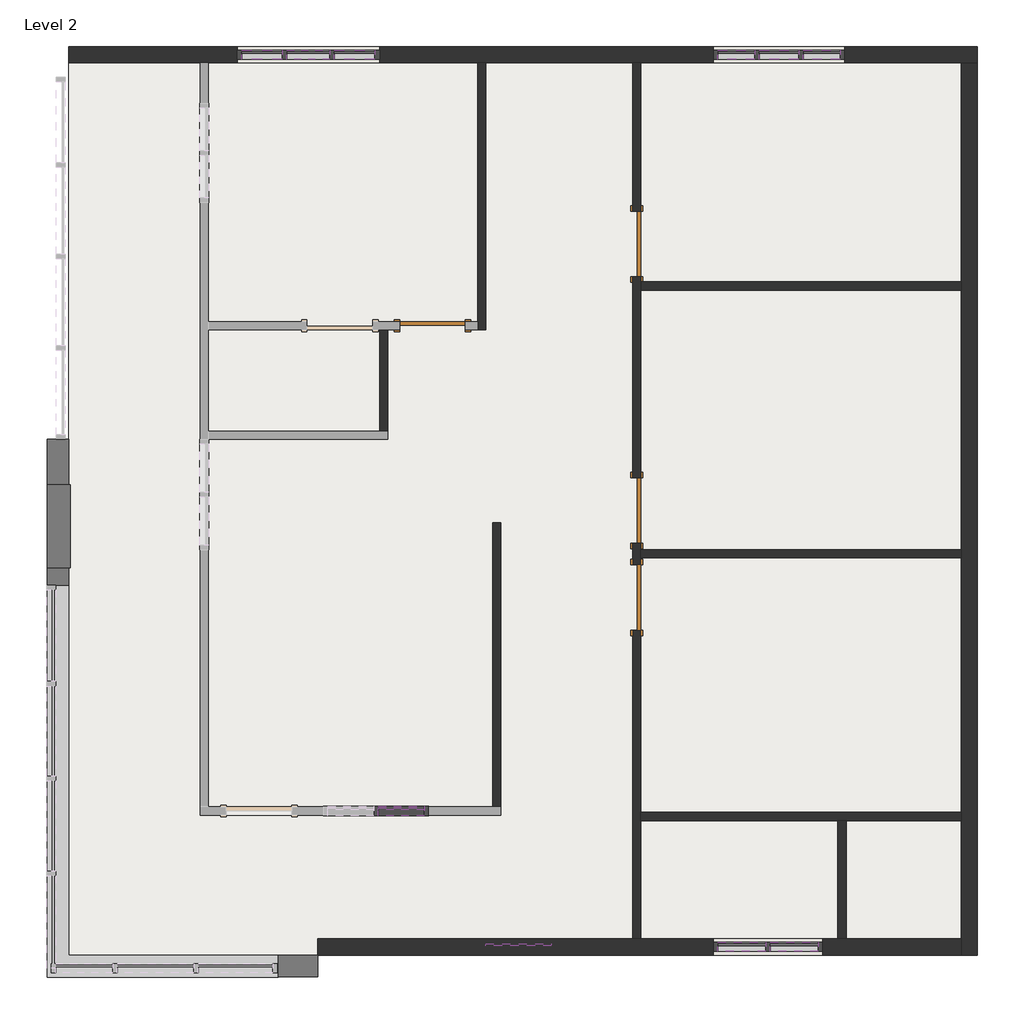
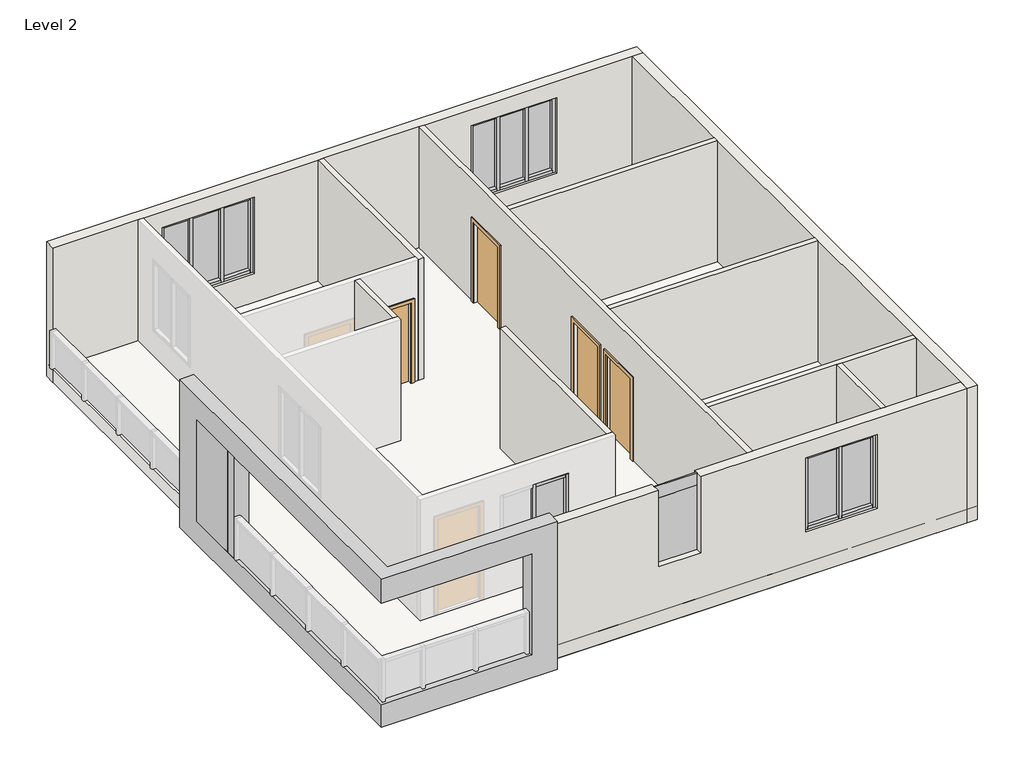
# One storey, part 2 of 2: 31 members, 11 plates, 11 walls, 4 doors, 1 proxy, 1 roof.
"""IFC4 building model written with IfcOpenShell, lengths in millimetres."""

from ifc_helpers import new_model, si_unit, frame, origin, place, context, project, spatial, polyline, outline, extrude, faceted_brep, transform, mapped, element, save
from components import generic_models_2_generic_models_2_8568020c, door_305aa2a5, door_e5f9f3c4, member_0b7646a3, member_a400357f, member_04adda39, member_21317375, member_6ffa5180, member_a980948f, member_e59d77c9, member_427039da, member_6f432376, member_fceb641e, member_70523b0d, member_c33c434a, member_3b0b484b, member_6d86f51b, system_panel_glazed_d508df5b, system_panel_glazed_080605c3, system_panel_glazed_66fd639c, system_panel_glazed_47f9b868, system_panel_glazed_7d7b3bbd, system_panel_glazed_3397605a, system_panel_glazed_23092caa, system_panel_glazed_25c2e5f5

model = new_model("IFC4")

# Units and contexts
model_context = context("Model", 3, world=origin())
ifc_project = project(units=[si_unit("LENGTHUNIT", "METRE", prefix="MILLI")], contexts=[model_context])

# Site, building, storey
site = spatial("IfcSite", under=ifc_project)
building = spatial("IfcBuilding", under=site)
storey = spatial("IfcBuildingStorey", under=building, Name="Level 2", Elevation=3048.0)

# Proxy
placement = place(None, origin())
generic_models_2_generic_models_2_shape = generic_models_2_generic_models_2_8568020c(model_context)
element("IfcBuildingElementProxy", 1, Name="Generic Models 2 : Generic Models 2", ObjectType="Generic Models 2 : Generic Models 2", at=placement, inside=storey, context=model_context, shape_type="MappedRepresentation", body=[
    mapped(generic_models_2_generic_models_2_shape, transform((0.0, 0.0, 0.0), x_axis=(1.0, 0.0, 0.0), y_axis=(0.0, 1.0, 0.0), z_axis=(0.0, 0.0, 1.0))),
])

# Doors
door_shape = door_305aa2a5(model_context)
element("IfcDoor", 2, ObjectType="Single-Flush : 36\" x 84\"", at=placement, inside=storey, context=model_context, shape_type="MappedRepresentation", body=[
    mapped(door_shape, transform((-12359.0003587, -8894.9526331, 3048.0), x_axis=(0.0, 1.0, 0.0), y_axis=(-1.0, 0.0, 0.0), z_axis=(0.0, 0.0, 1.0))),
])
door_2_shape = door_e5f9f3c4(model_context)
element("IfcDoor", 3, ObjectType="Single-Flush : 36\" x 84\"", at=placement, inside=storey, context=model_context, shape_type="MappedRepresentation", body=[
    mapped(door_2_shape, transform((-15200.6253587, -5110.3526331, 3048.0), x_axis=(1.0, 0.0, 0.0), y_axis=(0.0, 1.0, 0.0), z_axis=(0.0, 0.0, 1.0))),
])
element("IfcDoor", 4, ObjectType="Single-Flush : 36\" x 84\"", at=placement, inside=storey, context=model_context, shape_type="MappedRepresentation", body=[
    mapped(door_2_shape, transform((-12359.0003587, -3973.7026331, 3048.0), x_axis=(0.0, -1.0, 0.0), y_axis=(1.0, 0.0, 0.0), z_axis=(0.0, 0.0, 1.0))),
])
element("IfcDoor", 5, ObjectType="Single-Flush : 36\" x 84\"", at=placement, inside=storey, context=model_context, shape_type="MappedRepresentation", body=[
    mapped(door_2_shape, transform((-12359.0003587, -7682.1026331, 3048.0), x_axis=(0.0, -1.0, 0.0), y_axis=(1.0, 0.0, 0.0), z_axis=(0.0, 0.0, 1.0))),
])

# Members
member_shape = member_0b7646a3(model_context)
element("IfcMember", 6, ObjectType="Rectangular Mullion : 2.5\" x 5\" rectangular", at=placement, inside=storey, context=model_context, shape_type="MappedRepresentation", body=[
    mapped(member_shape, transform((-10714.3503587, -1338.4526331, 5725.9797172), x_axis=(0.0, 0.0, 1.0), y_axis=(0.0, -1.0, 0.0), z_axis=(1.0, 0.0, 0.0))),
])
element("IfcMember", 7, ObjectType="Rectangular Mullion : 2.5\" x 5\" rectangular", at=placement, inside=storey, context=model_context, shape_type="MappedRepresentation", body=[
    mapped(member_shape, transform((-9526.9003587, -1338.4526331, 5725.9797172), x_axis=(0.0, 0.0, 1.0), y_axis=(0.0, -1.0, 0.0), z_axis=(1.0, 0.0, 0.0))),
])
element("IfcMember", 8, ObjectType="Rectangular Mullion : 2.5\" x 5\" rectangular", at=placement, inside=storey, context=model_context, shape_type="MappedRepresentation", body=[
    mapped(member_shape, transform((-10041.2503587, -1338.4526331, 4005.1947307), x_axis=(0.0, 0.0, -1.0), y_axis=(0.0, -1.0, 0.0), z_axis=(-1.0, 0.0, 0.0))),
])
element("IfcMember", 9, ObjectType="Rectangular Mullion : 2.5\" x 5\" rectangular", at=placement, inside=storey, context=model_context, shape_type="MappedRepresentation", body=[
    mapped(member_shape, transform((-11228.7003587, -1338.4526331, 4005.1947307), x_axis=(0.0, 0.0, -1.0), y_axis=(0.0, -1.0, 0.0), z_axis=(-1.0, 0.0, 0.0))),
])
member_2_shape = member_a400357f(model_context)
element("IfcMember", 10, ObjectType="Rectangular Mullion : 2.5\" x 5\" rectangular", at=placement, inside=storey, context=model_context, shape_type="MappedRepresentation", body=[
    mapped(member_2_shape, transform((-16632.5503587, -1338.4526331, 5732.407438), x_axis=(0.0, 0.0, 1.0), y_axis=(0.0, -1.0, 0.0), z_axis=(1.0, 0.0, 0.0))),
])
element("IfcMember", 11, ObjectType="Rectangular Mullion : 2.5\" x 5\" rectangular", at=placement, inside=storey, context=model_context, shape_type="MappedRepresentation", body=[
    mapped(member_2_shape, transform((-17229.4503587, -1338.4526331, 4006.4763266), x_axis=(0.0, 0.0, -1.0), y_axis=(0.0, -1.0, 0.0), z_axis=(-1.0, 0.0, 0.0))),
])
member_3_shape = member_04adda39(model_context)
element("IfcMember", 12, ObjectType="Rectangular Mullion : 2.5\" x 5\" rectangular", at=placement, inside=storey, context=model_context, shape_type="MappedRepresentation", body=[
    mapped(member_3_shape, transform((-15318.1003587, -11866.7526331, 5586.8732654), x_axis=(0.0, 0.0, 1.0), y_axis=(0.0, -1.0, 0.0), z_axis=(1.0, 0.0, 0.0))),
])
member_4_shape = member_21317375(model_context)
element("IfcMember", 13, ObjectType="Rectangular Mullion : 2.5\" x 5\" rectangular", at=placement, inside=storey, context=model_context, shape_type="MappedRepresentation", body=[
    mapped(member_4_shape, transform((-15988.0253587, -11866.7526331, 4227.0998045), x_axis=(1.0, 0.0, 0.0), y_axis=(0.0, -1.0, 0.0), z_axis=(0.0, 0.0, -1.0))),
])
element("IfcMember", 14, ObjectType="Rectangular Mullion : 2.5\" x 5\" rectangular", at=placement, inside=storey, context=model_context, shape_type="MappedRepresentation", body=[
    mapped(member_3_shape, transform((-15956.2753587, -11866.7526331, 4227.0998045), x_axis=(0.0, 0.0, -1.0), y_axis=(0.0, -1.0, 0.0), z_axis=(-1.0, 0.0, 0.0))),
])
member_5_shape = member_6ffa5180(model_context)
element("IfcMember", 15, ObjectType="Rectangular Mullion : 2.5\" x 5\" rectangular", at=placement, inside=storey, context=model_context, shape_type="MappedRepresentation", body=[
    mapped(member_5_shape, transform((-15254.6003587, -11866.7526331, 4227.0998045), x_axis=(1.0, 0.0, 0.0), y_axis=(0.0, -1.0, 0.0), z_axis=(0.0, 0.0, -1.0))),
])
member_6_shape = member_a980948f(model_context)
element("IfcMember", 16, ObjectType="Rectangular Mullion : 2.5\" x 5\" rectangular", at=placement, inside=storey, context=model_context, shape_type="MappedRepresentation", body=[
    mapped(member_6_shape, transform((-10104.7503587, -1338.4526331, 5725.9797172), x_axis=(0.0, 0.0, 1.0), y_axis=(0.0, -1.0, 0.0), z_axis=(1.0, 0.0, 0.0))),
])
member_7_shape = member_e59d77c9(model_context)
element("IfcMember", 17, ObjectType="Rectangular Mullion : 2.5\" x 5\" rectangular", at=placement, inside=storey, context=model_context, shape_type="MappedRepresentation", body=[
    mapped(member_7_shape, transform((-10682.6003587, -1338.4526331, 4005.1947307), x_axis=(1.0, 0.0, 0.0), y_axis=(0.0, -1.0, 0.0), z_axis=(0.0, 0.0, -1.0))),
])
element("IfcMember", 18, ObjectType="Rectangular Mullion : 2.5\" x 5\" rectangular", at=placement, inside=storey, context=model_context, shape_type="MappedRepresentation", body=[
    mapped(member_7_shape, transform((-10073.0003587, -1338.4526331, 4005.1947307), x_axis=(1.0, 0.0, 0.0), y_axis=(0.0, -1.0, 0.0), z_axis=(0.0, 0.0, -1.0))),
])
element("IfcMember", 19, ObjectType="Rectangular Mullion : 2.5\" x 5\" rectangular", at=placement, inside=storey, context=model_context, shape_type="MappedRepresentation", body=[
    mapped(member_6_shape, transform((-10650.8503587, -1338.4526331, 4005.1947307), x_axis=(0.0, 0.0, -1.0), y_axis=(0.0, -1.0, 0.0), z_axis=(-1.0, 0.0, 0.0))),
])
member_8_shape = member_427039da(model_context)
element("IfcMember", 20, ObjectType="Rectangular Mullion : 2.5\" x 5\" rectangular", at=placement, inside=storey, context=model_context, shape_type="MappedRepresentation", body=[
    mapped(member_8_shape, transform((-11292.2003587, -1338.4526331, 5725.9797172), x_axis=(-1.0, 0.0, 0.0), y_axis=(0.0, -1.0, 0.0), z_axis=(0.0, 0.0, 1.0))),
])
element("IfcMember", 21, ObjectType="Rectangular Mullion : 2.5\" x 5\" rectangular", at=placement, inside=storey, context=model_context, shape_type="MappedRepresentation", body=[
    mapped(member_8_shape, transform((-9463.4003587, -1338.4526331, 4005.1947307), x_axis=(1.0, 0.0, 0.0), y_axis=(0.0, -1.0, 0.0), z_axis=(0.0, 0.0, -1.0))),
])
member_9_shape = member_6f432376(model_context)
element("IfcMember", 22, ObjectType="Rectangular Mullion : 2.5\" x 5\" rectangular", at=placement, inside=storey, context=model_context, shape_type="MappedRepresentation", body=[
    mapped(member_9_shape, transform((-17292.9503587, -1338.4526331, 5732.407438), x_axis=(0.0, 0.0, 1.0), y_axis=(0.0, -1.0, 0.0), z_axis=(1.0, 0.0, 0.0))),
])
element("IfcMember", 23, ObjectType="Rectangular Mullion : 2.5\" x 5\" rectangular", at=placement, inside=storey, context=model_context, shape_type="MappedRepresentation", body=[
    mapped(member_9_shape, transform((-16003.9003587, -1338.4526331, 5732.407438), x_axis=(0.0, 0.0, 1.0), y_axis=(0.0, -1.0, 0.0), z_axis=(1.0, 0.0, 0.0))),
])
member_10_shape = member_fceb641e(model_context)
element("IfcMember", 24, ObjectType="Rectangular Mullion : 2.5\" x 5\" rectangular", at=placement, inside=storey, context=model_context, shape_type="MappedRepresentation", body=[
    mapped(member_10_shape, transform((-16600.8003587, -1338.4526331, 4006.4763266), x_axis=(1.0, 0.0, 0.0), y_axis=(0.0, -1.0, 0.0), z_axis=(0.0, 0.0, -1.0))),
])
element("IfcMember", 25, ObjectType="Rectangular Mullion : 2.5\" x 5\" rectangular", at=placement, inside=storey, context=model_context, shape_type="MappedRepresentation", body=[
    mapped(member_10_shape, transform((-17261.2003587, -1338.4526331, 4006.4763266), x_axis=(1.0, 0.0, 0.0), y_axis=(0.0, -1.0, 0.0), z_axis=(0.0, 0.0, -1.0))),
])
element("IfcMember", 26, ObjectType="Rectangular Mullion : 2.5\" x 5\" rectangular", at=placement, inside=storey, context=model_context, shape_type="MappedRepresentation", body=[
    mapped(member_9_shape, transform((-16569.0503587, -1338.4526331, 4006.4763266), x_axis=(0.0, 0.0, -1.0), y_axis=(0.0, -1.0, 0.0), z_axis=(-1.0, 0.0, 0.0))),
])
element("IfcMember", 27, ObjectType="Rectangular Mullion : 2.5\" x 5\" rectangular", at=placement, inside=storey, context=model_context, shape_type="MappedRepresentation", body=[
    mapped(member_9_shape, transform((-17858.1003587, -1338.4526331, 4006.4763266), x_axis=(0.0, 0.0, -1.0), y_axis=(0.0, -1.0, 0.0), z_axis=(-1.0, 0.0, 0.0))),
])
member_11_shape = member_70523b0d(model_context)
element("IfcMember", 28, ObjectType="Rectangular Mullion : 2.5\" x 5\" rectangular", at=placement, inside=storey, context=model_context, shape_type="MappedRepresentation", body=[
    mapped(member_11_shape, transform((-17921.6003587, -1338.4526331, 5732.407438), x_axis=(-1.0, 0.0, 0.0), y_axis=(0.0, -1.0, 0.0), z_axis=(0.0, 0.0, 1.0))),
])
element("IfcMember", 29, ObjectType="Rectangular Mullion : 2.5\" x 5\" rectangular", at=placement, inside=storey, context=model_context, shape_type="MappedRepresentation", body=[
    mapped(member_11_shape, transform((-15940.4003587, -1338.4526331, 4006.4763266), x_axis=(1.0, 0.0, 0.0), y_axis=(0.0, -1.0, 0.0), z_axis=(0.0, 0.0, -1.0))),
])
member_12_shape = member_c33c434a(model_context)
element("IfcMember", 30, ObjectType="Rectangular Mullion : 2.5\" x 5\" rectangular", at=placement, inside=storey, context=model_context, shape_type="MappedRepresentation", body=[
    mapped(member_12_shape, transform((-10561.9503587, -13759.0526331, 5725.9797172), x_axis=(0.0, 0.0, 1.0), y_axis=(0.0, -1.0, 0.0), z_axis=(1.0, 0.0, 0.0))),
])
element("IfcMember", 31, ObjectType="Rectangular Mullion : 2.5\" x 5\" rectangular", at=placement, inside=storey, context=model_context, shape_type="MappedRepresentation", body=[
    mapped(member_12_shape, transform((-9831.7003587, -13759.0526331, 5725.9797172), x_axis=(0.0, 0.0, 1.0), y_axis=(0.0, -1.0, 0.0), z_axis=(1.0, 0.0, 0.0))),
])
element("IfcMember", 32, ObjectType="Rectangular Mullion : 2.5\" x 5\" rectangular", at=placement, inside=storey, context=model_context, shape_type="MappedRepresentation", body=[
    mapped(member_12_shape, transform((-10498.4503587, -13759.0526331, 4050.5645472), x_axis=(0.0, 0.0, -1.0), y_axis=(0.0, -1.0, 0.0), z_axis=(-1.0, 0.0, 0.0))),
])
element("IfcMember", 33, ObjectType="Rectangular Mullion : 2.5\" x 5\" rectangular", at=placement, inside=storey, context=model_context, shape_type="MappedRepresentation", body=[
    mapped(member_12_shape, transform((-11228.7003587, -13759.0526331, 4050.5645472), x_axis=(0.0, 0.0, -1.0), y_axis=(0.0, -1.0, 0.0), z_axis=(-1.0, 0.0, 0.0))),
])
member_13_shape = member_3b0b484b(model_context)
element("IfcMember", 34, ObjectType="Rectangular Mullion : 2.5\" x 5\" rectangular", at=placement, inside=storey, context=model_context, shape_type="MappedRepresentation", body=[
    mapped(member_13_shape, transform((-10530.2003587, -13759.0526331, 4050.5645472), x_axis=(1.0, 0.0, 0.0), y_axis=(0.0, -1.0, 0.0), z_axis=(0.0, 0.0, -1.0))),
])
member_14_shape = member_6d86f51b(model_context)
element("IfcMember", 35, ObjectType="Rectangular Mullion : 2.5\" x 5\" rectangular", at=placement, inside=storey, context=model_context, shape_type="MappedRepresentation", body=[
    mapped(member_14_shape, transform((-9768.2003587, -13759.0526331, 4050.5645472), x_axis=(1.0, 0.0, 0.0), y_axis=(0.0, -1.0, 0.0), z_axis=(0.0, 0.0, -1.0))),
])
element("IfcMember", 36, ObjectType="Rectangular Mullion : 2.5\" x 5\" rectangular", at=placement, inside=storey, context=model_context, shape_type="MappedRepresentation", body=[
    mapped(member_14_shape, transform((-11292.2003587, -13759.0526331, 5725.9797172), x_axis=(-1.0, 0.0, 0.0), y_axis=(0.0, -1.0, 0.0), z_axis=(0.0, 0.0, 1.0))),
])

# Plates
system_panel_glazed_shape = system_panel_glazed_d508df5b(model_context)
element("IfcPlate", 37, ObjectType="System Panel : Glazed", at=placement, inside=storey, context=model_context, shape_type="MappedRepresentation", body=[
    mapped(system_panel_glazed_shape, transform((-15637.1878587, -11866.7526331, 4290.5998045), x_axis=(1.0, 0.0, 0.0), y_axis=(0.0, 1.0, 0.0), z_axis=(0.0, 0.0, 1.0))),
])
system_panel_glazed_2_shape = system_panel_glazed_080605c3(model_context)
element("IfcPlate", 38, ObjectType="System Panel : Glazed", at=placement, inside=storey, context=model_context, shape_type="MappedRepresentation", body=[
    mapped(system_panel_glazed_2_shape, transform((-10971.5253587, -1338.4526331, 4068.6947307), x_axis=(1.0, 0.0, 0.0), y_axis=(0.0, 1.0, 0.0), z_axis=(0.0, 0.0, 1.0))),
])
element("IfcPlate", 39, ObjectType="System Panel : Glazed", at=placement, inside=storey, context=model_context, shape_type="MappedRepresentation", body=[
    mapped(system_panel_glazed_2_shape, transform((-9784.0753587, -1338.4526331, 4068.6947307), x_axis=(1.0, 0.0, 0.0), y_axis=(0.0, 1.0, 0.0), z_axis=(0.0, 0.0, 1.0))),
])
system_panel_glazed_3_shape = system_panel_glazed_66fd639c(model_context)
element("IfcPlate", 40, ObjectType="System Panel : Glazed", at=placement, inside=storey, context=model_context, shape_type="MappedRepresentation", body=[
    mapped(system_panel_glazed_3_shape, transform((-10377.8003587, -1338.4526331, 4068.6947307), x_axis=(1.0, 0.0, 0.0), y_axis=(0.0, 1.0, 0.0), z_axis=(0.0, 0.0, 1.0))),
])
system_panel_glazed_4_shape = system_panel_glazed_47f9b868(model_context)
element("IfcPlate", 41, ObjectType="System Panel : Glazed", at=placement, inside=storey, context=model_context, shape_type="MappedRepresentation", body=[
    mapped(system_panel_glazed_4_shape, transform((-17575.5253587, -1338.4526331, 4069.9763266), x_axis=(1.0, 0.0, 0.0), y_axis=(0.0, 1.0, 0.0), z_axis=(0.0, 0.0, 1.0))),
])
element("IfcPlate", 42, ObjectType="System Panel : Glazed", at=placement, inside=storey, context=model_context, shape_type="MappedRepresentation", body=[
    mapped(system_panel_glazed_4_shape, transform((-16286.4753587, -1338.4526331, 4069.9763266), x_axis=(1.0, 0.0, 0.0), y_axis=(0.0, 1.0, 0.0), z_axis=(0.0, 0.0, 1.0))),
])
system_panel_glazed_5_shape = system_panel_glazed_7d7b3bbd(model_context)
element("IfcPlate", 43, ObjectType="System Panel : Glazed", at=placement, inside=storey, context=model_context, shape_type="MappedRepresentation", body=[
    mapped(system_panel_glazed_5_shape, transform((-16931.0003587, -1338.4526331, 4069.9763266), x_axis=(1.0, 0.0, 0.0), y_axis=(0.0, 1.0, 0.0), z_axis=(0.0, 0.0, 1.0))),
])
system_panel_glazed_6_shape = system_panel_glazed_3397605a(model_context)
element("IfcPlate", 44, ObjectType="System Panel : Glazed", at=placement, inside=storey, context=model_context, shape_type="MappedRepresentation", body=[
    mapped(system_panel_glazed_6_shape, transform((-14003.6503587, -13759.0526331, 4361.7460332), x_axis=(1.0, 0.0, 0.0), y_axis=(0.0, 1.0, 0.0), z_axis=(0.0, 0.0, 1.0))),
])
system_panel_glazed_7_shape = system_panel_glazed_23092caa(model_context)
element("IfcPlate", 45, ObjectType="System Panel : Glazed", at=placement, inside=storey, context=model_context, shape_type="MappedRepresentation", body=[
    mapped(system_panel_glazed_7_shape, transform((-14003.6503587, -13759.0526331, 5816.6), x_axis=(1.0, 0.0, 0.0), y_axis=(0.0, 1.0, 0.0), z_axis=(0.0, 0.0, 1.0))),
])
system_panel_glazed_8_shape = system_panel_glazed_25c2e5f5(model_context)
element("IfcPlate", 46, ObjectType="System Panel : Glazed", at=placement, inside=storey, context=model_context, shape_type="MappedRepresentation", body=[
    mapped(system_panel_glazed_8_shape, transform((-10895.3253587, -13759.0526331, 4114.0645472), x_axis=(1.0, 0.0, 0.0), y_axis=(0.0, 1.0, 0.0), z_axis=(0.0, 0.0, 1.0))),
])
element("IfcPlate", 47, ObjectType="System Panel : Glazed", at=placement, inside=storey, context=model_context, shape_type="MappedRepresentation", body=[
    mapped(system_panel_glazed_8_shape, transform((-10165.0753587, -13759.0526331, 4114.0645472), x_axis=(1.0, 0.0, 0.0), y_axis=(0.0, 1.0, 0.0), z_axis=(0.0, 0.0, 1.0))),
])

# Roof
element("IfcRoof", 48, ObjectType="Generic - 12\"", at=placement, inside=storey, context=model_context, shape_type="SweptSolid", body=[
    extrude(outline(polyline([(-20264.7503587, -1224.1526331), (-7615.5503587, -1224.1526331), (-7615.5503587, -13873.3526331), (-20264.7503587, -13873.3526331), (-20264.7503587, -1224.1526331)])), frame((0.0, 0.0, 3048.0), z_axis=(0.0, 0.0, 1.0), x_axis=(1.0, 0.0, 0.0)), (0.0, 0.0, 1.0), 304.8),
])

# Walls
element("IfcWall", 49, ObjectType="4.5\"", at=placement, inside=storey, context=model_context, shape_type="Brep", body=[
    faceted_brep([(-12301.8503587, -8437.7526331, 5181.6), (-12301.8503587, -8437.7526331, 3048.0), (-12301.8503587, -8342.5026331, 3048.0), (-12301.8503587, -8228.2026331, 3048.0), (-12301.8503587, -8139.3026331, 3048.0), (-12301.8503587, -8139.3026331, 5181.6), (-12301.8503587, -7224.9026331, 5181.6), (-12301.8503587, -7224.9026331, 3048.0), (-12301.8503587, -4615.0526331, 3048.0), (-12301.8503587, -4500.7526331, 3048.0), (-12301.8503587, -4430.9026331, 3048.0), (-12301.8503587, -4430.9026331, 5181.6), (-12301.8503587, -3516.5026331, 5181.6), (-12301.8503587, -3516.5026331, 3048.0), (-12301.8503587, -1452.7526331, 3048.0), (-12301.8503587, -1452.7526331, 6096.0), (-12301.8503587, -4500.7526331, 6096.0), (-12301.8503587, -4615.0526331, 6096.0), (-12301.8503587, -8228.2026331, 6096.0), (-12301.8503587, -8342.5026331, 6096.0), (-12301.8503587, -11885.8026331, 6096.0), (-12301.8503587, -12000.1026331, 6096.0), (-12301.8503587, -13644.7526331, 6096.0), (-12301.8503587, -13644.7526331, 3048.0), (-12301.8503587, -12000.1026331, 3048.0), (-12301.8503587, -11885.8026331, 3048.0), (-12301.8503587, -9352.1526331, 3048.0), (-12301.8503587, -9352.1526331, 5181.6), (-12416.1503587, -8139.3026331, 3048.0), (-12416.1503587, -8437.7526331, 3048.0), (-12416.1503587, -8437.7526331, 5181.6), (-12416.1503587, -9352.1526331, 5181.6), (-12416.1503587, -9352.1526331, 3048.0), (-12416.1503587, -13644.7526331, 3048.0), (-12416.1503587, -13644.7526331, 6096.0), (-12416.1503587, -1452.7526331, 6096.0), (-12416.1503587, -1452.7526331, 3048.0), (-12416.1503587, -3516.5026331, 3048.0), (-12416.1503587, -3516.5026331, 5181.6), (-12416.1503587, -4430.9026331, 5181.6), (-12416.1503587, -4430.9026331, 3048.0), (-12416.1503587, -7224.9026331, 3048.0), (-12416.1503587, -7224.9026331, 5181.6), (-12416.1503587, -8139.3026331, 5181.6)], [[[0, 1, 2, 3, 4, 5, 6, 7, 8, 9, 10, 11, 12, 13, 14, 15, 16, 17, 18, 19, 20, 21, 22, 23, 24, 25, 26, 27]], [[28, 29, 30, 31, 32, 33, 34, 35, 36, 37, 38, 39, 40, 41, 42, 43]], [[37, 36, 14, 13]], [[41, 40, 10, 9, 8, 7]], [[26, 25, 24, 23, 33, 32]], [[4, 3, 2, 1, 29, 28]], [[22, 21, 20, 19, 18, 17, 16, 15, 35, 34]], [[15, 14, 36, 35]], [[11, 10, 40, 39]], [[12, 11, 39, 38]], [[13, 12, 38, 37]], [[5, 4, 28, 43]], [[6, 5, 43, 42]], [[7, 6, 42, 41]], [[30, 29, 1, 0]], [[31, 30, 0, 27]], [[32, 31, 27, 26]], [[23, 22, 34, 33]]]),
])
element("IfcWall", 50, ObjectType="4.5\"", at=placement, inside=storey, context=model_context, shape_type="SweptSolid", body=[
    extrude(outline(polyline([(-7844.1503587, -4615.0526331), (-12301.8503587, -4615.0526331), (-12301.8503587, -4500.7526331), (-7844.1503587, -4500.7526331), (-7844.1503587, -4615.0526331)])), frame((0.0, 0.0, 3048.0), z_axis=(0.0, 0.0, 1.0), x_axis=(1.0, 0.0, 0.0)), (0.0, 0.0, 1.0), 3048.0),
])
element("IfcWall", 51, ObjectType="4.5\"", at=placement, inside=storey, context=model_context, shape_type="Brep", body=[
    faceted_brep([(-12301.8503587, -12000.1026331, 3048.0), (-9558.6503587, -12000.1026331, 3048.0), (-9444.3503587, -12000.1026331, 3048.0), (-7844.1503587, -12000.1026331, 3048.0), (-7844.1503587, -12000.1026331, 6096.0), (-9444.3503587, -12000.1026331, 6096.0), (-9558.6503587, -12000.1026331, 6096.0), (-12301.8503587, -12000.1026331, 6096.0), (-12301.8503587, -11885.8026331, 3048.0), (-12301.8503587, -11885.8026331, 6096.0), (-7844.1503587, -11885.8026331, 6096.0), (-7844.1503587, -11885.8026331, 3048.0)], [[[0, 1, 2, 3, 4, 5, 6, 7]], [[8, 9, 10, 11]], [[3, 2, 1, 0, 8, 11]], [[7, 6, 5, 4, 10, 9]], [[4, 3, 11, 10]], [[0, 7, 9, 8]]]),
])
element("IfcWall", 52, ObjectType="4.5\"", at=placement, inside=storey, context=model_context, shape_type="SweptSolid", body=[
    extrude(outline(polyline([(-9558.6503587, -13644.7526331), (-9558.6503587, -12000.1026331), (-9444.3503587, -12000.1026331), (-9444.3503587, -13644.7526331), (-9558.6503587, -13644.7526331)])), frame((0.0, 0.0, 3048.0), z_axis=(0.0, 0.0, 1.0), x_axis=(1.0, 0.0, 0.0)), (0.0, 0.0, 1.0), 3048.0),
])
element("IfcWall", 53, ObjectType="4.5\"", at=placement, inside=storey, context=model_context, shape_type="Brep", body=[
    faceted_brep([(-14575.1503587, -1452.7526331, 3048.0), (-14575.1503587, -5053.2026331, 3048.0), (-14575.1503587, -5167.5026331, 3048.0), (-14575.1503587, -5167.5026331, 6096.0), (-14575.1503587, -5053.2026331, 6096.0), (-14575.1503587, -1452.7526331, 6096.0), (-14460.8503587, -1452.7526331, 3048.0), (-14460.8503587, -1452.7526331, 6096.0), (-14460.8503587, -5167.5026331, 6096.0), (-14460.8503587, -5167.5026331, 3048.0)], [[[0, 1, 2, 3, 4, 5]], [[6, 7, 8, 9]], [[2, 1, 0, 6, 9]], [[5, 4, 3, 8, 7]], [[0, 5, 7, 6]], [[3, 2, 9, 8]]]),
])
element("IfcWall", 54, ObjectType="4.5\"", at=placement, inside=storey, context=model_context, shape_type="SweptSolid", body=[
    extrude(outline(polyline([(-15826.1003587, -5167.5026331), (-15826.1003587, -6577.2026331), (-15940.4003587, -6577.2026331), (-15940.4003587, -5167.5026331), (-15826.1003587, -5167.5026331)])), frame((0.0, 0.0, 3048.0), z_axis=(0.0, 0.0, 1.0), x_axis=(1.0, 0.0, 0.0)), (0.0, 0.0, 1.0), 3048.0),
])
element("IfcWall", 55, ObjectType="4.5\"", at=placement, inside=storey, context=model_context, shape_type="SweptSolid", body=[
    extrude(outline(polyline([(-14251.3003587, -7853.5526331), (-14251.3003587, -11809.6026331), (-14365.6003587, -11809.6026331), (-14365.6003587, -7853.5526331), (-14251.3003587, -7853.5526331)])), frame((0.0, 0.0, 3048.0), z_axis=(0.0, 0.0, 1.0), x_axis=(1.0, 0.0, 0.0)), (0.0, 0.0, 1.0), 3048.0),
])
element("IfcWall", 56, ObjectType="4.5\"", at=placement, inside=storey, context=model_context, shape_type="SweptSolid", body=[
    extrude(outline(polyline([(-7844.1503587, -8342.5026331), (-12301.8503587, -8342.5026331), (-12301.8503587, -8228.2026331), (-7844.1503587, -8228.2026331), (-7844.1503587, -8342.5026331)])), frame((0.0, 0.0, 3048.0), z_axis=(0.0, 0.0, 1.0), x_axis=(1.0, 0.0, 0.0)), (0.0, 0.0, 1.0), 3048.0),
])
element("IfcWall", 57, ObjectType="9\"", at=placement, inside=storey, context=model_context, shape_type="Brep", body=[
    faceted_brep([(-20264.7503587, -1452.7526331, 3048.0), (-18435.9503587, -1452.7526331, 3048.0), (-18321.6503587, -1452.7526331, 3048.0), (-14575.1503587, -1452.7526331, 3048.0), (-14460.8503587, -1452.7526331, 3048.0), (-12416.1503587, -1452.7526331, 3048.0), (-12301.8503587, -1452.7526331, 3048.0), (-7844.1503587, -1452.7526331, 3048.0), (-7615.5503587, -1452.7526331, 3048.0), (-7615.5503587, -1452.7526331, 6096.0), (-7844.1503587, -1452.7526331, 6096.0), (-12301.8503587, -1452.7526331, 6096.0), (-12416.1503587, -1452.7526331, 6096.0), (-14460.8503587, -1452.7526331, 6096.0), (-14575.1503587, -1452.7526331, 6096.0), (-18321.6503587, -1452.7526331, 6096.0), (-18435.9503587, -1452.7526331, 6096.0), (-20264.7503587, -1452.7526331, 6096.0), (-17921.6003587, -1452.7526331, 4006.4763266), (-17921.6003587, -1452.7526331, 5732.407438), (-15940.4003587, -1452.7526331, 5732.407438), (-15940.4003587, -1452.7526331, 4006.4763266), (-11292.2003587, -1452.7526331, 4005.1947307), (-11292.2003587, -1452.7526331, 5725.9797172), (-9463.4003587, -1452.7526331, 5725.9797172), (-9463.4003587, -1452.7526331, 4005.1947307), (-7615.5503587, -1224.1526331, 3048.0), (-20264.7503587, -1224.1526331, 3048.0), (-20264.7503587, -1224.1526331, 6096.0), (-7615.5503587, -1224.1526331, 6096.0), (-17921.6003587, -1224.1526331, 5732.407438), (-17921.6003587, -1224.1526331, 4006.4763266), (-15940.4003587, -1224.1526331, 4006.4763266), (-15940.4003587, -1224.1526331, 5732.407438), (-11292.2003587, -1224.1526331, 5725.9797172), (-11292.2003587, -1224.1526331, 4005.1947307), (-9463.4003587, -1224.1526331, 4005.1947307), (-9463.4003587, -1224.1526331, 5725.9797172)], [[[0, 1, 2, 3, 4, 5, 6, 7, 8, 9, 10, 11, 12, 13, 14, 15, 16, 17], [18, 19, 20, 21], [22, 23, 24, 25]], [[26, 27, 28, 29], [30, 31, 32, 33], [34, 35, 36, 37]], [[8, 7, 6, 5, 4, 3, 2, 1, 0, 27, 26]], [[17, 16, 15, 14, 13, 12, 11, 10, 9, 29, 28]], [[0, 17, 28, 27]], [[9, 8, 26, 29]], [[18, 31, 30, 19]], [[19, 30, 33, 20]], [[20, 33, 32, 21]], [[31, 18, 21, 32]], [[22, 35, 34, 23]], [[23, 34, 37, 24]], [[36, 25, 24, 37]], [[35, 22, 25, 36]]]),
])
element("IfcWall", 58, ObjectType="9\"", at=placement, inside=storey, context=model_context, shape_type="Brep", body=[
    faceted_brep([(-7844.1503587, -1452.7526331, 3048.0), (-7844.1503587, -4500.7526331, 3048.0), (-7844.1503587, -4615.0526331, 3048.0), (-7844.1503587, -8228.2026331, 3048.0), (-7844.1503587, -8342.5026331, 3048.0), (-7844.1503587, -11885.8026331, 3048.0), (-7844.1503587, -12000.1026331, 3048.0), (-7844.1503587, -13644.7526331, 3048.0), (-7844.1503587, -13873.3526331, 3048.0), (-7844.1503587, -13873.3526331, 6096.0), (-7844.1503587, -13644.7526331, 6096.0), (-7844.1503587, -12000.1026331, 6096.0), (-7844.1503587, -11885.8026331, 6096.0), (-7844.1503587, -8342.5026331, 6096.0), (-7844.1503587, -8228.2026331, 6096.0), (-7844.1503587, -4615.0526331, 6096.0), (-7844.1503587, -4500.7526331, 6096.0), (-7844.1503587, -1452.7526331, 6096.0), (-7615.5503587, -1452.7526331, 3048.0), (-7615.5503587, -1452.7526331, 6096.0), (-7615.5503587, -13873.3526331, 6096.0), (-7615.5503587, -13873.3526331, 3048.0)], [[[0, 1, 2, 3, 4, 5, 6, 7, 8, 9, 10, 11, 12, 13, 14, 15, 16, 17]], [[18, 19, 20, 21]], [[8, 7, 6, 5, 4, 3, 2, 1, 0, 18, 21]], [[17, 16, 15, 14, 13, 12, 11, 10, 9, 20, 19]], [[0, 17, 19, 18]], [[9, 8, 21, 20]]]),
])
element("IfcWall", 59, ObjectType="9\"", at=placement, inside=storey, context=model_context, shape_type="Brep", body=[
    faceted_brep([(-7844.1503587, -13644.7526331, 3048.0), (-9444.3503587, -13644.7526331, 3048.0), (-9558.6503587, -13644.7526331, 3048.0), (-12301.8503587, -13644.7526331, 3048.0), (-12416.1503587, -13644.7526331, 3048.0), (-16797.6503587, -13644.7526331, 3048.0), (-16797.6503587, -13644.7526331, 6096.0), (-14460.8503587, -13644.7526331, 6096.0), (-14460.8503587, -13644.7526331, 4361.7460332), (-13546.4503587, -13644.7526331, 4361.7460332), (-13546.4503587, -13644.7526331, 6096.0), (-12416.1503587, -13644.7526331, 6096.0), (-12301.8503587, -13644.7526331, 6096.0), (-9558.6503587, -13644.7526331, 6096.0), (-9444.3503587, -13644.7526331, 6096.0), (-7844.1503587, -13644.7526331, 6096.0), (-11292.2003587, -13644.7526331, 5725.9797172), (-11292.2003587, -13644.7526331, 4050.5645472), (-9768.2003587, -13644.7526331, 4050.5645472), (-9768.2003587, -13644.7526331, 5725.9797172), (-16797.6503587, -13873.3526331, 3048.0), (-7844.1503587, -13873.3526331, 3048.0), (-7844.1503587, -13873.3526331, 6096.0), (-13546.4503587, -13873.3526331, 6096.0), (-13546.4503587, -13873.3526331, 4361.7460332), (-14460.8503587, -13873.3526331, 4361.7460332), (-14460.8503587, -13873.3526331, 6096.0), (-16797.6503587, -13873.3526331, 6096.0), (-11292.2003587, -13873.3526331, 4050.5645472), (-11292.2003587, -13873.3526331, 5725.9797172), (-9768.2003587, -13873.3526331, 5725.9797172), (-9768.2003587, -13873.3526331, 4050.5645472)], [[[0, 1, 2, 3, 4, 5, 6, 7, 8, 9, 10, 11, 12, 13, 14, 15], [16, 17, 18, 19]], [[20, 21, 22, 23, 24, 25, 26, 27], [28, 29, 30, 31]], [[5, 4, 3, 2, 1, 0, 21, 20]], [[6, 5, 20, 27]], [[6, 27, 26, 7]], [[22, 15, 14, 13, 12, 11, 10, 23]], [[0, 15, 22, 21]], [[25, 8, 7, 26]], [[9, 24, 23, 10]], [[8, 25, 24, 9]], [[28, 17, 16, 29]], [[29, 16, 19, 30]], [[30, 19, 18, 31]], [[17, 28, 31, 18]]]),
])

save(model, "model.ifc")

# Revit data of these elements
# Type "Single-Flush : 36\" x 84\""
#   Type Mark = "1"
#   Construction Type Id = "MDOOR"
#   Assembly Code = "C1020"
#   Analytic Construction = "Metal"
#   Thickness = 0' - 2"
#   Heat Transfer Coefficient (U) = 0.651978 BTU/(h·ft²·°F)
#   Height = 7' - 0"
#   Trim Projection Ext = 0' - 1"
#   Trim Projection Int = 0' - 1"
#   Trim Width = 0' - 3"
#   Width = 3' - 0"
#   Define Thermal Properties by = 1
#   Define Thermal Properties by = 1
#   Door Material = Door - Panel
#   Frame Material = Door - Frame
#   Visual Light Transmittance = 0
#   Solar Heat Gain Coefficient = 0
#   Function = (empty or 0)
#   Wall Closure = (empty or 0)
# Type "Rectangular Mullion : 2.5\" x 5\" rectangular"
#   built-in parameter 1007304 = 0.416667 (stored number, unit not read)
#   built-in parameter 1007301 = 0.104167 (stored number, unit not read)
#   built-in parameter 1007300 = 0.104167 (stored number, unit not read)
# Type "System Panel : Glazed"
#   Construction Type Id = "GSP4R"
#   Analytic Construction = "1/8 in Pilkington single glazing"
#   Visual Light Transmittance = 0.9
#   Solar Heat Gain Coefficient = 0.86
#   Heat Transfer Coefficient (U) = 1.18115 BTU/(h·ft²·°F)
#   Define Thermal Properties by = 1
# Type "Generic - 12\""
#   Assembly Code = "B1020"
#   Layers, outside or top first: 1' - 0" no material (function 1)
# Type "4.5\""
#   Assembly Code = "B2010"
#   Layers, outside or top first: 0' - 4 1/2" no material (function 1)
# Type "9\""
#   Assembly Code = "B2010"
#   Layers, outside or top first: 0' - 9" no material (function 1)
# Element 1 (IfcBuildingElementProxy, "Generic Models 2 : Generic Models 2")
#   Phase Created = New Construction
# Elements 2, 3, 4, 5 (IfcDoor, "Single-Flush : 36\" x 84\"")
#   Phase Created = New Construction
#   Materials on its faces: "Door - Frame", "Door - Panel"
# Elements 6, 7, 8, 9, 10, 11, 12, 13, 14, 15, 16, 17, 18, 19, 20, 21, 22, 23, 24, 25, 26, 27, 28, 29, 30, 31, 32, 33, 34, 35, 36 (IfcMember, "Rectangular Mullion : 2.5\" x 5\" rectangular")
#   Phase Created = New Construction
#   Materials on its faces: "Aluminum"
# Elements 37, 38, 39, 40, 41, 42, 43, 44, 45, 46, 47 (IfcPlate, "System Panel : Glazed")
#   Phase Created = New Construction
#   Materials on its faces: "Glass"
# Element 48 (IfcRoof, "Generic - 12\"")
#   built-in parameter 1001705 = 11 (stored number, unit not read)
#   built-in parameter 1001710 = 33615
#   Phase Created = New Construction
#   Materials on its faces: "Default Roof"
# Elements 49, 50, 51, 52, 53, 54, 55, 56 (IfcWall, "4.5\"")
#   Top Offset = 0' - 0"
#   Base Offset = 0' - 0"
#   Unconnected Height = 10' - 0"
#   wall height = 10' - 0"
#   Phase Created = New Construction
#   Base Constraint = Level 2
#   Materials on its faces: "Default Wall"
# Elements 57, 58, 59 (IfcWall, "9\"")
#   Top Offset = 0' - 0"
#   Base Offset = 0' - 0"
#   Unconnected Height = 10' - 0"
#   wall height = 10' - 0"
#   Phase Created = New Construction
#   Base Constraint = Level 2
#   Materials on its faces: "Default Wall"
# Materials
#   "Door - Panel": class "Wood", colour RGB 210 159 95, transparency 0, Cost = 0
#   "Door - Frame": colour RGB 118 70 51, transparency 0, Cost = 0
#   "Aluminum": class "Metal", colour RGB 247 247 247, transparency 0, Description = "Aluminum 6061", Cost = 0
#   "Glass": class "Glass", colour RGB 0 128 192, transparency 0.75, Description = "Soda Lime Glass", Cost = 0
#   "Default Roof": colour RGB 88 101 114, transparency 0, Cost = 0
#   "Default Wall": colour RGB 128 128 128, transparency 0, Cost = 0
